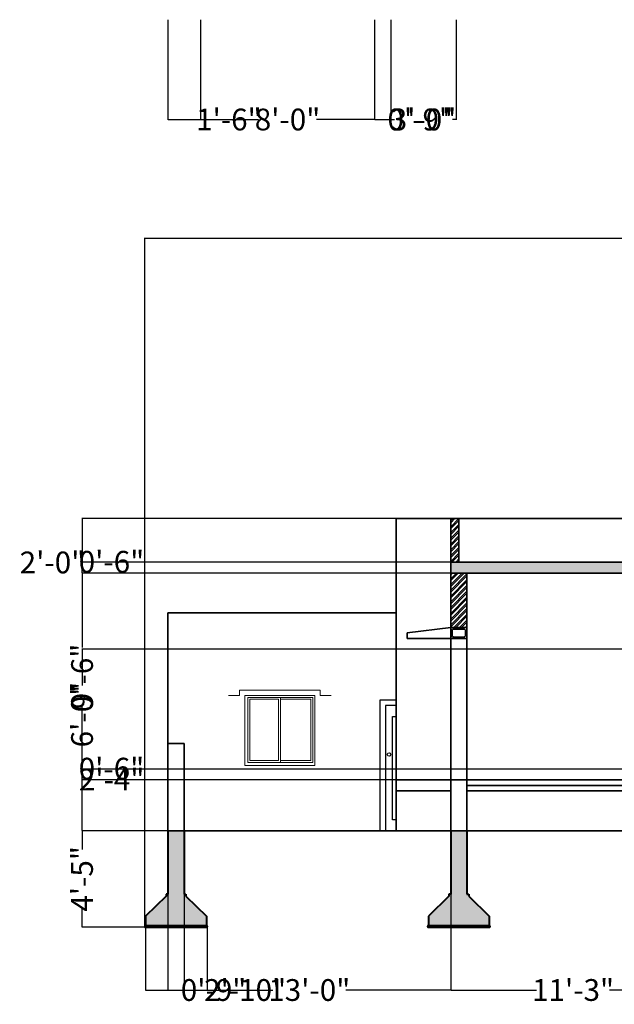
# Model space of a CAD drawing. Units: inches. Extents: x 1146 to 2917, y 889 to 2437.
# Tile 1 of 13: x 1223 to 1551, y 889 to 1432. Entities that reach past the tile are written whole.
import ezdxf

# ---------------------------------------------------------------- set-up
doc = ezdxf.new("R2010")
doc.units = ezdxf.units.IN
doc.header["$MEASUREMENT"] = 0
for name, color, linetype, lineweight in [('A-ANNO-DIMS', 2, 'Continuous', 18), ('A-SECT', 7, 'Continuous', 35), ('A-SECT-PATT', 8, 'Continuous', 13), ('door', 10, 'Continuous', 25), ('S-FNDN', 7, 'Continuous', 40), ('window', 5, 'Continuous', 18)]:
    doc.layers.add(name, color=color, linetype=linetype, lineweight=lineweight)
doc.styles.get("Standard").update_dxf_attribs({"font": 'arial.ttf'})
doc.dimstyles.get("Standard").update_dxf_attribs({"dimtxt": 12, "dimasz": 0.18, "dimexe": 0.18, "dimexo": 0.0625, "dimgap": 0.09, "dimtad": 0, "dimtoh": 1, "dimdec": 1, "dimzin": 0, "dimdsep": 46, "dimlunit": 4, "dimtxsty": 'Standard', "dimcen": 0.09, "dimadec": 0, "dimazin": 0, "dimtfac": 1, "dimtdec": 1, "dimtofl": 0, "dimtmove": 0, "dimatfit": 3, "dimfxl": 1, "dimtolj": 1, "dimtzin": 0, "dimarcsym": 0})
pattern_1 = [(50, (0, 0), (2.1517805, -0.1882564), [0.225, -2.475]), (355, (0, 0), (-0.416254, 2.2565764), [0.18, -1.98]), (100.45144, (0.1793, -0.0157), (1.7355265, 2.06832), [0.1912206, -2.1034263]), (46.1842, (0, 0.6), (3.201724, -0.496558), [0.3375, -3.7125]), (96.63564, (0.2668, 0.5586), (2.803986, 2.922356), [0.286831, -3.1551413]), (351.18416, (0, 0.6), (2.803986, 2.922356), [0.27, -2.97]), (21, (0.3, 0.45), (1.7907212, -1.2078567), [0.225, -2.475]), (326, (0.3, 0.45), (0.729946, 2.1754501), [0.18, -1.98]), (71.45144, (0.4492, 0.3493), (2.5206671, 0.9675935), [0.1912206, -2.1034263]), (37.5, (0, 0), (0.03647957, 0.99868156), [0, -1.956, 0, -2.01, 0, -1.9875]), (7.5, (0, 0), (0.7892086, 1.18323514), [0, -1.146, 0, -1.911, 0, -0.7575]), (327.5, (-0.669, 0), (1.6014673, -0.06766462), [0, -0.75, 0, -2.34, 0, -3.105]), (317.5, (-0.969, 0), (1.7495585, 0.30031495), [0, -0.975, 0, -1.554, 0, -2.205])]

# ---------------------------------------------------------------- blocks, each defined once
blk = doc.blocks.new('*D141')
at = {"layer": 'A-ANNO-DIMS', "color": 0, "lineweight": -2, "transparency": 16777216}
for p, q in [((1292.5, 931.94), (1292.5, 1311.7)), ((1292.68, 1311.52), (1597.13, 1311.52)), ((1970.95, 1311.52), (1666.5, 1311.52)), ((1971.13, 1277.03), (1971.13, 1311.7))]:
    blk.add_line(p, q, dxfattribs=at)
at = {"layer": 'A-ANNO-DIMS', "color": 0, "transparency": 16777216}
for points in [[(1292.68, 1311.55), (1292.68, 1311.49), (1292.5, 1311.52)], [(1970.95, 1311.55), (1970.95, 1311.49), (1971.13, 1311.52)]]:
    blk.add_solid(points, dxfattribs=at)
at = {"layer": 'Defpoints', "color": 0, "transparency": 16777216}
for p in [(1971.13, 1311.52), (1971.13, 1276.97), (1292.5, 931.87)]:
    blk.add_point(p, dxfattribs=at)
at = {"layer": 'A-ANNO-DIMS', "color": 0, "transparency": 16777216, "insert": (1631.82, 1311.52), "char_height": 12, "attachment_point": 5}
blk.add_mtext('\\A1;56\'-6 1/2"', dxfattribs=at)
blk = doc.blocks.new('*D143')
at = {"layer": 'A-ANNO-DIMS', "color": 0, "lineweight": -2, "transparency": 16777216}
for p, q in [((1431.07, 1012.97), (1257.62, 1012.97)), ((1257.8, 1012.97), (1257.8, 1013.15)), ((1257.8, 1013.15), (1257.98, 1013.15)), ((1257.8, 985.15), (1257.8, 1012.79)), ((1431.07, 984.97), (1257.62, 984.97))]:
    blk.add_line(p, q, dxfattribs=at)
at = {"layer": 'A-ANNO-DIMS', "color": 0, "transparency": 16777216}
for points in [[(1257.77, 1012.79), (1257.83, 1012.79), (1257.8, 1012.97)], [(1257.77, 985.15), (1257.83, 985.15), (1257.8, 984.97)]]:
    blk.add_solid(points, dxfattribs=at)
at = {"layer": 'Defpoints', "color": 0, "transparency": 16777216}
for p in [(1257.8, 1012.97), (1431.13, 1012.97), (1431.13, 984.97)]:
    blk.add_point(p, dxfattribs=at)
at = {"layer": 'A-ANNO-DIMS', "color": 0, "transparency": 16777216, "insert": (1274.12, 1013.15), "char_height": 12, "attachment_point": 5}
blk.add_mtext('\\A1;2\'-4"', dxfattribs=at)
blk = doc.blocks.new('*D144')
at = {"layer": 'A-ANNO-DIMS', "color": 0, "lineweight": -2, "transparency": 16777216}
for p, q in [((1470.07, 1126.97), (1257.62, 1126.97)), ((1257.8, 1126.79), (1257.8, 1086.01)), ((1257.8, 1013.15), (1257.8, 1053.93)), ((1470.07, 1012.97), (1257.62, 1012.97))]:
    blk.add_line(p, q, dxfattribs=at)
at = {"layer": 'A-ANNO-DIMS', "color": 0, "transparency": 16777216}
for points in [[(1257.77, 1126.79), (1257.83, 1126.79), (1257.8, 1126.97)], [(1257.77, 1013.15), (1257.83, 1013.15), (1257.8, 1012.97)]]:
    blk.add_solid(points, dxfattribs=at)
at = {"layer": 'Defpoints', "color": 0, "transparency": 16777216}
for p in [(1470.13, 1126.97), (1257.8, 1012.97), (1470.13, 1012.97)]:
    blk.add_point(p, dxfattribs=at)
at = {"layer": 'A-ANNO-DIMS', "color": 0, "transparency": 16777216, "insert": (1257.8, 1069.97), "char_height": 12, "attachment_point": 5, "rotation": 90}
blk.add_mtext('\\A1;9\'-6"', dxfattribs=at)
blk = doc.blocks.new('*D145')
at = {"layer": 'A-ANNO-DIMS', "color": 0, "lineweight": -2, "transparency": 16777216}
for p, q in [((1461.07, 1156.97), (1257.62, 1156.97)), ((1257.8, 1156.79), (1257.8, 1133.15)), ((1461.07, 1132.97), (1257.62, 1132.97)), ((1257.8, 1132.79), (1257.62, 1132.79)), ((1257.8, 1132.97), (1257.8, 1132.79))]:
    blk.add_line(p, q, dxfattribs=at)
at = {"layer": 'A-ANNO-DIMS', "color": 0, "transparency": 16777216}
for points in [[(1257.77, 1156.79), (1257.83, 1156.79), (1257.8, 1156.97)], [(1257.77, 1133.15), (1257.83, 1133.15), (1257.8, 1132.97)]]:
    blk.add_solid(points, dxfattribs=at)
at = {"layer": 'Defpoints', "color": 0, "transparency": 16777216}
for p in [(1461.13, 1156.97), (1257.8, 1132.97), (1461.13, 1132.97)]:
    blk.add_point(p, dxfattribs=at)
at = {"layer": 'A-ANNO-DIMS', "color": 0, "transparency": 16777216, "insert": (1241.48, 1132.79), "char_height": 12, "attachment_point": 5}
blk.add_mtext('\\A1;2\'-0"', dxfattribs=at)
blk = doc.blocks.new('*D146')
at = {"layer": 'A-ANNO-DIMS', "color": 0, "lineweight": -2, "transparency": 16777216}
for p, q in [((1305.13, 984.9), (1305.13, 897)), ((1461.13, 984.9), (1461.13, 897)), ((1305.31, 897.18), (1363, 897.18)), ((1460.95, 897.18), (1403.27, 897.18))]:
    blk.add_line(p, q, dxfattribs=at)
at = {"layer": 'A-ANNO-DIMS', "color": 0, "transparency": 16777216}
for points in [[(1305.31, 897.21), (1305.31, 897.15), (1305.13, 897.18)], [(1460.95, 897.21), (1460.95, 897.15), (1461.13, 897.18)]]:
    blk.add_solid(points, dxfattribs=at)
at = {"layer": 'Defpoints', "color": 0, "transparency": 16777216}
for p in [(1305.13, 984.97), (1461.13, 984.97), (1461.13, 897.18)]:
    blk.add_point(p, dxfattribs=at)
at = {"layer": 'A-ANNO-DIMS', "color": 0, "transparency": 16777216, "insert": (1383.13, 897.18), "char_height": 12, "attachment_point": 5}
blk.add_mtext('\\A1;13\'-0"', dxfattribs=at)
blk = doc.blocks.new('*D147')
at = {"layer": 'A-ANNO-DIMS', "color": 0, "lineweight": -2, "transparency": 16777216}
for p, q in [((1461.13, 984.9), (1461.13, 897)), ((1596.13, 984.9), (1596.13, 897)), ((1461.31, 897.18), (1508.5, 897.18)), ((1595.95, 897.18), (1548.77, 897.18))]:
    blk.add_line(p, q, dxfattribs=at)
at = {"layer": 'A-ANNO-DIMS', "color": 0, "transparency": 16777216}
for points in [[(1461.31, 897.21), (1461.31, 897.15), (1461.13, 897.18)], [(1595.95, 897.21), (1595.95, 897.15), (1596.13, 897.18)]]:
    blk.add_solid(points, dxfattribs=at)
at = {"layer": 'Defpoints', "color": 0, "transparency": 16777216}
for p in [(1461.13, 984.97), (1596.13, 984.97), (1596.13, 897.18)]:
    blk.add_point(p, dxfattribs=at)
at = {"layer": 'A-ANNO-DIMS', "color": 0, "transparency": 16777216, "insert": (1528.63, 897.18), "char_height": 12, "attachment_point": 5}
blk.add_mtext('\\A1;11\'-3"', dxfattribs=at)
blk = doc.blocks.new('*D150')
at = {"layer": 'A-ANNO-DIMS', "color": 0, "lineweight": -2, "transparency": 16777216}
for p, q in [((1305.07, 984.97), (1257.62, 984.97)), ((1257.8, 984.79), (1257.8, 974.7)), ((1257.8, 932.05), (1257.8, 942.14)), ((1292.44, 931.87), (1257.62, 931.87))]:
    blk.add_line(p, q, dxfattribs=at)
at = {"layer": 'A-ANNO-DIMS', "color": 0, "transparency": 16777216}
for points in [[(1257.77, 984.79), (1257.83, 984.79), (1257.8, 984.97)], [(1257.77, 932.05), (1257.83, 932.05), (1257.8, 931.87)]]:
    blk.add_solid(points, dxfattribs=at)
at = {"layer": 'Defpoints', "color": 0, "transparency": 16777216}
for p in [(1305.13, 984.97), (1257.8, 931.87), (1292.5, 931.87)]:
    blk.add_point(p, dxfattribs=at)
at = {"layer": 'A-ANNO-DIMS', "color": 0, "transparency": 16777216, "insert": (1257.8, 958.42), "char_height": 12, "attachment_point": 5, "rotation": 90}
blk.add_mtext('\\A1;4\'-5"', dxfattribs=at)
blk = doc.blocks.new('*D154')
at = {"layer": 'A-ANNO-DIMS', "color": 0, "lineweight": -2, "transparency": 16777216}
for p, q in [((1830.07, 1018.97), (1257.62, 1018.97)), ((1257.8, 1018.97), (1257.8, 1019.15)), ((1257.8, 1019.15), (1257.98, 1019.15)), ((1257.8, 1013.15), (1257.8, 1018.79)), ((1830.07, 1012.97), (1257.62, 1012.97))]:
    blk.add_line(p, q, dxfattribs=at)
at = {"layer": 'A-ANNO-DIMS', "color": 0, "transparency": 16777216}
for points in [[(1257.77, 1018.79), (1257.83, 1018.79), (1257.8, 1018.97)], [(1257.77, 1013.15), (1257.83, 1013.15), (1257.8, 1012.97)]]:
    blk.add_solid(points, dxfattribs=at)
at = {"layer": 'Defpoints', "color": 0, "transparency": 16777216}
for p in [(1257.8, 1018.97), (1830.13, 1018.97), (1830.13, 1012.97)]:
    blk.add_point(p, dxfattribs=at)
at = {"layer": 'A-ANNO-DIMS', "color": 0, "transparency": 16777216, "insert": (1274.02, 1019.15), "char_height": 12, "attachment_point": 5}
blk.add_mtext('\\A1;0\'-6"', dxfattribs=at)
blk = doc.blocks.new('*D157')
at = {"layer": 'A-ANNO-DIMS', "color": 0, "lineweight": -2, "transparency": 16777216}
for p, q in [((1830.07, 1084.97), (1257.62, 1084.97)), ((1257.8, 1084.79), (1257.8, 1065.04)), ((1257.8, 1013.15), (1257.8, 1032.89)), ((1830.07, 1012.97), (1257.62, 1012.97))]:
    blk.add_line(p, q, dxfattribs=at)
at = {"layer": 'A-ANNO-DIMS', "color": 0, "transparency": 16777216}
for points in [[(1257.77, 1084.79), (1257.83, 1084.79), (1257.8, 1084.97)], [(1257.77, 1013.15), (1257.83, 1013.15), (1257.8, 1012.97)]]:
    blk.add_solid(points, dxfattribs=at)
at = {"layer": 'Defpoints', "color": 0, "transparency": 16777216}
for p in [(1257.8, 1084.97), (1830.13, 1084.97), (1830.13, 1012.97)]:
    blk.add_point(p, dxfattribs=at)
at = {"layer": 'A-ANNO-DIMS', "color": 0, "transparency": 16777216, "insert": (1257.8, 1048.97), "char_height": 12, "attachment_point": 5, "rotation": 90}
blk.add_mtext('\\A1;6\'-0"', dxfattribs=at)
blk = doc.blocks.new('*D158')
at = {"layer": 'A-ANNO-DIMS', "color": 0, "lineweight": -2, "transparency": 16777216}
for p, q in [((1461.07, 1132.97), (1257.62, 1132.97)), ((1257.8, 1132.97), (1257.8, 1133.15)), ((1257.8, 1133.15), (1257.98, 1133.15)), ((1257.8, 1127.15), (1257.8, 1132.79)), ((1461.07, 1126.97), (1257.62, 1126.97))]:
    blk.add_line(p, q, dxfattribs=at)
at = {"layer": 'A-ANNO-DIMS', "color": 0, "transparency": 16777216}
for points in [[(1257.77, 1132.79), (1257.83, 1132.79), (1257.8, 1132.97)], [(1257.77, 1127.15), (1257.83, 1127.15), (1257.8, 1126.97)]]:
    blk.add_solid(points, dxfattribs=at)
at = {"layer": 'Defpoints', "color": 0, "transparency": 16777216}
for p in [(1257.8, 1132.97), (1461.13, 1132.97), (1461.13, 1126.97)]:
    blk.add_point(p, dxfattribs=at)
at = {"layer": 'A-ANNO-DIMS', "color": 0, "transparency": 16777216, "insert": (1274.02, 1133.15), "char_height": 12, "attachment_point": 5}
blk.add_mtext('\\A1;0\'-6"', dxfattribs=at)
blk = doc.blocks.new('*D159')
at = {"layer": 'A-ANNO-DIMS', "color": 0, "lineweight": -2, "transparency": 16777216}
for p, q in [((1292.85, 932.16), (1292.85, 897)), ((1326.77, 931.81), (1326.77, 897)), ((1293.03, 897.18), (1326.59, 897.18)), ((1326.77, 897.18), (1326.95, 897.18))]:
    blk.add_line(p, q, dxfattribs=at)
at = {"layer": 'A-ANNO-DIMS', "color": 0, "transparency": 16777216}
for points in [[(1293.03, 897.21), (1293.03, 897.15), (1292.85, 897.18)], [(1326.59, 897.21), (1326.59, 897.15), (1326.77, 897.18)]]:
    blk.add_solid(points, dxfattribs=at)
at = {"layer": 'Defpoints', "color": 0, "transparency": 16777216}
for p in [(1292.85, 932.23), (1326.77, 931.87), (1326.77, 897.18)]:
    blk.add_point(p, dxfattribs=at)
at = {"layer": 'A-ANNO-DIMS', "color": 0, "transparency": 16777216, "insert": (1347.75, 897.18), "char_height": 12, "attachment_point": 5}
blk.add_mtext('\\A1;2\'-10"', dxfattribs=at)
blk = doc.blocks.new('*D160')
at = {"layer": 'A-ANNO-DIMS', "color": 0, "lineweight": -2, "transparency": 16777216}
for p, q in [((1305.13, 984.9), (1305.13, 897)), ((1314.13, 984.9), (1314.13, 897)), ((1305.31, 897.18), (1313.95, 897.18)), ((1314.13, 897.18), (1314.31, 897.18))]:
    blk.add_line(p, q, dxfattribs=at)
at = {"layer": 'A-ANNO-DIMS', "color": 0, "transparency": 16777216}
for points in [[(1305.31, 897.21), (1305.31, 897.15), (1305.13, 897.18)], [(1313.95, 897.21), (1313.95, 897.15), (1314.13, 897.18)]]:
    blk.add_solid(points, dxfattribs=at)
at = {"layer": 'Defpoints', "color": 0, "transparency": 16777216}
for p in [(1305.13, 984.97), (1314.13, 984.97), (1314.13, 897.18)]:
    blk.add_point(p, dxfattribs=at)
at = {"layer": 'A-ANNO-DIMS', "color": 0, "transparency": 16777216, "insert": (1330.35, 897.18), "char_height": 12, "attachment_point": 5}
blk.add_mtext('\\A1;0\'-9"', dxfattribs=at)
blk = doc.blocks.new('*D162')
at = {"layer": 'A-ANNO-DIMS', "color": 0, "lineweight": -2, "transparency": 16777216}
for p, q in [((1305.13, 1431.83), (1305.13, 1376.71)), ((1323.13, 1431.83), (1323.13, 1376.71)), ((1305.31, 1376.89), (1322.95, 1376.89)), ((1323.13, 1376.89), (1323.31, 1376.89))]:
    blk.add_line(p, q, dxfattribs=at)
at = {"layer": 'A-ANNO-DIMS', "color": 0, "transparency": 16777216}
for points in [[(1305.31, 1376.92), (1305.31, 1376.86), (1305.13, 1376.89)], [(1322.95, 1376.92), (1322.95, 1376.86), (1323.13, 1376.89)]]:
    blk.add_solid(points, dxfattribs=at)
at = {"layer": 'Defpoints', "color": 0, "transparency": 16777216}
for p in [(1305.13, 1431.89), (1323.13, 1431.89), (1323.13, 1376.89)]:
    blk.add_point(p, dxfattribs=at)
at = {"layer": 'A-ANNO-DIMS', "color": 0, "transparency": 16777216, "insert": (1338.79, 1376.89), "char_height": 12, "attachment_point": 5}
blk.add_mtext('\\A1;1\'-6"', dxfattribs=at)
blk = doc.blocks.new('*D163')
at = {"layer": 'A-ANNO-DIMS', "color": 0, "lineweight": -2, "transparency": 16777216}
for p, q in [((1323.13, 1431.83), (1323.13, 1376.71)), ((1419.13, 1431.83), (1419.13, 1376.71)), ((1323.31, 1376.89), (1355.09, 1376.89)), ((1418.95, 1376.89), (1387.18, 1376.89))]:
    blk.add_line(p, q, dxfattribs=at)
at = {"layer": 'A-ANNO-DIMS', "color": 0, "transparency": 16777216}
for points in [[(1323.31, 1376.92), (1323.31, 1376.86), (1323.13, 1376.89)], [(1418.95, 1376.92), (1418.95, 1376.86), (1419.13, 1376.89)]]:
    blk.add_solid(points, dxfattribs=at)
at = {"layer": 'Defpoints', "color": 0, "transparency": 16777216}
for p in [(1323.13, 1431.89), (1419.13, 1431.89), (1419.13, 1376.89)]:
    blk.add_point(p, dxfattribs=at)
at = {"layer": 'A-ANNO-DIMS', "color": 0, "transparency": 16777216, "insert": (1371.13, 1376.89), "char_height": 12, "attachment_point": 5}
blk.add_mtext('\\A1;8\'-0"', dxfattribs=at)
blk = doc.blocks.new('*D164')
at = {"layer": 'A-ANNO-DIMS', "color": 0, "lineweight": -2, "transparency": 16777216}
for p, q in [((1419.13, 1431.83), (1419.13, 1376.71)), ((1428.13, 1431.83), (1428.13, 1376.71)), ((1419.31, 1376.89), (1427.95, 1376.89)), ((1428.13, 1376.89), (1428.31, 1376.89))]:
    blk.add_line(p, q, dxfattribs=at)
at = {"layer": 'A-ANNO-DIMS', "color": 0, "transparency": 16777216}
for points in [[(1419.31, 1376.92), (1419.31, 1376.86), (1419.13, 1376.89)], [(1427.95, 1376.92), (1427.95, 1376.86), (1428.13, 1376.89)]]:
    blk.add_solid(points, dxfattribs=at)
at = {"layer": 'Defpoints', "color": 0, "transparency": 16777216}
for p in [(1419.13, 1431.89), (1428.13, 1431.89), (1428.13, 1376.89)]:
    blk.add_point(p, dxfattribs=at)
at = {"layer": 'A-ANNO-DIMS', "color": 0, "transparency": 16777216, "insert": (1444.35, 1376.89), "char_height": 12, "attachment_point": 5}
blk.add_mtext('\\A1;0\'-9"', dxfattribs=at)
blk = doc.blocks.new('*D165')
at = {"layer": 'A-ANNO-DIMS', "color": 0, "lineweight": -2, "transparency": 16777216}
for p, q in [((1428.13, 1431.83), (1428.13, 1376.71)), ((1464.13, 1431.83), (1464.13, 1376.71)), ((1428.31, 1376.89), (1430.1, 1376.89)), ((1463.95, 1376.89), (1462.17, 1376.89))]:
    blk.add_line(p, q, dxfattribs=at)
at = {"layer": 'A-ANNO-DIMS', "color": 0, "transparency": 16777216}
for points in [[(1428.31, 1376.92), (1428.31, 1376.86), (1428.13, 1376.89)], [(1463.95, 1376.92), (1463.95, 1376.86), (1464.13, 1376.89)]]:
    blk.add_solid(points, dxfattribs=at)
at = {"layer": 'Defpoints', "color": 0, "transparency": 16777216}
for p in [(1428.13, 1431.89), (1464.13, 1431.89), (1464.13, 1376.89)]:
    blk.add_point(p, dxfattribs=at)
at = {"layer": 'A-ANNO-DIMS', "color": 0, "transparency": 16777216, "insert": (1446.13, 1376.89), "char_height": 12, "attachment_point": 5}
blk.add_mtext('\\A1;3\'-0"', dxfattribs=at)

msp = doc.modelspace()

# ---------------------------------------------------------------- hatches: boundary and pattern name
at = {"layer": 'A-SECT-PATT'}
h = msp.add_hatch(dxfattribs=at)
h.set_pattern_fill('ANSI32', color=256, scale=6)
h.paths.add_polyline_path([(1605.13, 1126.97), (1596.13, 1126.97), (1596.13, 1102.97), (1605.13, 1102.97)])
h.paths.add_polyline_path([(1794.13, 1126.97), (1785.13, 1126.97), (1785.13, 1102.97), (1794.13, 1102.97)])
h.paths.add_polyline_path([(1470.13, 1126.97), (1461.13, 1126.97), (1461.13, 1096.97), (1470.13, 1096.97)])
h.paths.add_polyline_path([(1461.13, 1132.97), (1465.63, 1132.97), (1465.63, 1156.97), (1461.13, 1156.97)])
h = msp.add_hatch(dxfattribs=at)
h.set_pattern_fill('AR-CONC', color=256, scale=0.3)
h.set_pattern_definition(pattern_1)
h.paths.add_polyline_path([(1856.99, 1126.97), (1856.99, 1132.97), (1461.13, 1132.97), (1461.13, 1126.97)])
h = msp.add_hatch(dxfattribs=at)
h.set_pattern_fill('AR-CONC', color=256, scale=0.3)
h.set_pattern_definition(pattern_1)
h.paths.add_polyline_path([(1315.13, 948.97), (1315.13, 949.97), (1314.13, 949.97), (1314.13, 984.97), (1305.13, 984.97), (1305.13, 949.97), (1304.13, 949.97), (1304.13, 948.97), (1292.85, 937.8), (1292.85, 932.73), (1326.42, 932.73), (1326.42, 937.8)])
h = msp.add_hatch(dxfattribs=at)
h.set_pattern_fill('AR-CONC', color=256, scale=0.3)
h.set_pattern_definition([(50, (156, 0), (2.1517805, -0.1882564), [0.225, -2.475]), (355, (156, 0), (-0.416254, 2.2565764), [0.18, -1.98]), (100.45144, (156.1793, -0.0157), (1.7355265, 2.06832), [0.1912206, -2.1034263]), (46.1842, (156, 0.6), (3.201724, -0.496558), [0.3375, -3.7125]), (96.63564, (156.2668, 0.5586), (2.803986, 2.922356), [0.286831, -3.155141]), (351.18416, (156, 0.6), (2.803986, 2.922356), [0.27, -2.97]), (21, (156.3, 0.45), (1.7907212, -1.2078567), [0.225, -2.475]), (326, (156.3, 0.45), (0.729946, 2.17545), [0.18, -1.98]), (71.45144, (156.4492, 0.3493), (2.520667, 0.9675935), [0.1912206, -2.1034263]), (37.5, (156, 0), (0.03647957, 0.99868156), [0, -1.956, 0, -2.01, 0, -1.9875]), (7.5, (156, 0), (0.7892086, 1.18323514), [0, -1.146, 0, -1.911, 0, -0.7575]), (327.5, (155.331, 0), (1.6014673, -0.0676646), [0, -0.75, 0, -2.34, 0, -3.105]), (317.5, (155.031, 0), (1.7495585, 0.300315), [0, -0.975, 0, -1.554, 0, -2.205])])
h.paths.add_polyline_path([(1471.13, 948.97), (1471.13, 949.97), (1470.13, 949.97), (1470.13, 984.97), (1461.13, 984.97), (1461.13, 949.97), (1460.13, 949.97), (1460.13, 948.97), (1448.85, 937.8), (1448.85, 932.73), (1482.42, 932.73), (1482.42, 937.8)])

# ---------------------------------------------------------------- linework, layer by layer
at = {"layer": 'A-SECT'}
for p, q in [((1461.13, 1156.97), (1431.13, 1156.97)), ((1431.13, 1132.97), (1431.13, 1156.97)), ((1461.13, 1156.97), (1785.13, 1156.97)), ((1461.13, 1126.97), (1461.13, 1156.97)), ((1465.63, 1132.97), (1465.63, 1156.97)), ((1431.13, 1132.97), (1431.13, 984.97)), ((1461.13, 1132.97), (1856.99, 1132.97)), ((1461.13, 984.97), (1461.13, 1126.97)), ((1461.13, 1126.97), (1856.99, 1126.97)), ((1470.13, 984.97), (1470.13, 1126.97)), ((1305.13, 984.97), (1305.13, 1104.97)), ((1305.13, 1104.97), (1431.13, 1104.97)), ((1437.13, 1093.97), (1461.13, 1096.97)), ((1470.13, 1096.97), (1461.13, 1096.97)), ((1437.13, 1090.97), (1437.13, 1093.97)), ((1461.13, 1090.97), (1437.13, 1090.97)), ((1470.13, 1090.97), (1461.13, 1090.97)), ((1305.13, 1032.97), (1314.13, 1032.97)), ((1314.13, 984.97), (1314.13, 1032.97)), ((1638.13, 1012.97), (1431.13, 1012.97)), ((1470.13, 1012.97), (1971.13, 1012.97)), ((1470.13, 1009.97), (1596.13, 1009.97)), ((1431.13, 1006.97), (1461.13, 1006.97)), ((1470.13, 1006.97), (1596.13, 1006.97)), ((1305.13, 984.97), (1314.13, 984.97)), ((1314.13, 984.97), (1461.13, 984.97)), ((1461.13, 984.97), (1971.13, 984.97))]:
    msp.add_line(p, q, dxfattribs=at)
msp.add_lwpolyline([(1462.92, 1096.05), (1468.31, 1096.05, -0.414214), (1469.31, 1095.05), (1469.31, 1092.71, -0.414214), (1468.31, 1091.71), (1462.92, 1091.71, -0.414214), (1461.92, 1092.71), (1461.92, 1095.05, -0.414214)], format="xyb", close=True, dxfattribs=at)
at = {"layer": 'door'}
for points in [[(1431.13, 1056.97), (1422.13, 1056.97), (1422.13, 984.97), (1425.13, 984.97)], [(1431.13, 1053.94), (1425.13, 1053.94), (1425.13, 984.97), (1455.13, 984.97)], [(1431.13, 990.97), (1429.13, 990.97), (1429.13, 1047.94), (1431.13, 1047.94)], [(1455.13, 984.97), (1458.13, 984.97)]]:
    msp.add_lwpolyline(points, dxfattribs=at)
msp.add_circle((1427.13, 1026.97), 1, dxfattribs=at)
at = {"layer": 'S-FNDN'}
for p, q in [((1305.13, 984.97), (1305.13, 949.97)), ((1314.13, 984.97), (1314.13, 949.97)), ((1461.13, 984.97), (1461.13, 949.97)), ((1470.13, 984.97), (1470.13, 949.97)), ((1305.13, 949.97), (1304.13, 949.97)), ((1304.13, 949.97), (1304.13, 948.97)), ((1314.13, 949.97), (1315.13, 949.97)), ((1315.13, 949.97), (1315.13, 948.97)), ((1461.13, 949.97), (1460.13, 949.97)), ((1460.13, 949.97), (1460.13, 948.97)), ((1470.13, 949.97), (1471.13, 949.97)), ((1471.13, 949.97), (1471.13, 948.97)), ((1304.13, 948.97), (1292.85, 937.8)), ((1315.13, 948.97), (1326.42, 937.8)), ((1460.13, 948.97), (1448.85, 937.8)), ((1471.13, 948.97), (1482.42, 937.8)), ((1292.85, 937.8), (1292.85, 932.73)), ((1326.42, 937.8), (1326.42, 932.73)), ((1448.85, 937.8), (1448.85, 932.73)), ((1482.42, 937.8), (1482.42, 932.73)), ((1292.85, 932.73), (1326.42, 932.73)), ((1292.85, 931.73), (1326.42, 931.73)), ((1448.85, 932.73), (1482.42, 932.73)), ((1448.85, 931.73), (1482.42, 931.73))]:
    msp.add_line(p, q, dxfattribs=at)
for centre, start, end in [((1292.85, 932.23), 90, 270), ((1326.42, 932.23), 270, 90), ((1448.85, 932.23), 90, 270), ((1482.42, 932.23), 270, 90)]:
    msp.add_arc(centre, 0.5, start, end, dxfattribs=at)
at = {"layer": 'window'}
for p, q in [((1344.63, 1059.47), (1338.63, 1059.47)), ((1349.26, 1022.6), (1349.26, 1058.45)), ((1349.26, 1058.45), (1367.19, 1058.45)), ((1367.19, 1022.6), (1367.19, 1058.45)), ((1367.19, 1058.45), (1385.12, 1058.45)), ((1385.12, 1058.45), (1385.12, 1022.6)), ((1389.13, 1059.47), (1395.13, 1059.47)), ((1367.19, 1022.6), (1349.26, 1022.6)), ((1385.12, 1022.6), (1367.19, 1022.6))]:
    msp.add_line(p, q, dxfattribs=at)
for points in [[(1389.13, 1059.47), (1389.13, 1062.47), (1344.63, 1062.47), (1344.63, 1059.47)], [(1366.11, 1057.37), (1366.11, 1023.68), (1350.35, 1023.68), (1350.35, 1057.37), (1366.11, 1057.37)], [(1367.19, 1057.37), (1384.03, 1057.37), (1384.03, 1023.68), (1367.19, 1023.68)]]:
    msp.add_lwpolyline(points, dxfattribs=at)
msp.add_lwpolyline([(1347.63, 1020.97), (1386.13, 1020.97), (1386.13, 1059.47), (1347.63, 1059.47)], close=True, dxfattribs=at)

# ---------------------------------------------------------------- dimensions: what is measured, and where the dimension line sits
at = {"layer": 'A-ANNO-DIMS'}
for base, p1, p2, picture, middle in [((1323.13, 1376.89), (1305.13, 1431.89), (1323.13, 1431.89), '*D162', (1338.79, 1376.89)), ((1419.13, 1376.89), (1323.13, 1431.89), (1419.13, 1431.89), '*D163', (1371.13, 1376.89)), ((1428.13, 1376.89), (1419.13, 1431.89), (1428.13, 1431.89), '*D164', (1444.35, 1376.89)), ((1464.13, 1376.89), (1428.13, 1431.89), (1464.13, 1431.89), '*D165', (1446.13, 1376.89)), ((1971.13, 1311.52), (1292.5, 931.87), (1971.13, 1276.97), '*D141', (1631.82, 1311.52)), ((1461.13, 897.18), (1305.13, 984.97), (1461.13, 984.97), '*D146', (1383.13, 897.18)), ((1314.13, 897.18), (1305.13, 984.97), (1314.13, 984.97), '*D160', (1330.35, 897.18)), ((1596.13, 897.18), (1461.13, 984.97), (1596.13, 984.97), '*D147', (1528.63, 897.18)), ((1326.77, 897.18), (1292.85, 932.23), (1326.77, 931.87), '*D159', (1347.75, 897.18))]:
    dim = msp.add_linear_dim(base=base, p1=p1, p2=p2, dimstyle='Standard', override={"dimdec": 1, "dimlfac": 1, "dimrnd": 0, "dimzin": 1, "dimdsep": 46, "dimlunit": 4, "dimfrac": 2}, dxfattribs=at)
    dim.commit()
    dim.dimension.update_dxf_attribs({"geometry": picture, "text_midpoint": middle})
for base, p1, p2, picture, middle in [((1257.8, 1132.97), (1461.13, 1156.97), (1461.13, 1132.97), '*D145', (1241.48, 1132.79)), ((1257.8, 1132.97), (1461.13, 1126.97), (1461.13, 1132.97), '*D158', (1274.02, 1133.15)), ((1257.8, 1012.97), (1470.13, 1126.97), (1470.13, 1012.97), '*D144', (1257.8, 1069.97)), ((1257.8, 1084.97), (1830.13, 1012.97), (1830.13, 1084.97), '*D157', (1257.8, 1048.97)), ((1257.8, 1018.97), (1830.13, 1012.97), (1830.13, 1018.97), '*D154', (1274.02, 1019.15)), ((1257.8, 1012.97), (1431.13, 984.97), (1431.13, 1012.97), '*D143', (1274.12, 1013.15)), ((1257.8, 931.87), (1305.13, 984.97), (1292.5, 931.87), '*D150', (1257.8, 958.42))]:
    dim = msp.add_linear_dim(base=base, p1=p1, p2=p2, angle=90, dimstyle='Standard', override={"dimdec": 1, "dimlfac": 1, "dimrnd": 0, "dimzin": 1, "dimdsep": 46, "dimlunit": 4, "dimfrac": 2}, dxfattribs=at)
    dim.commit()
    dim.dimension.update_dxf_attribs({"geometry": picture, "text_midpoint": middle})

doc.saveas('drawing.dxf')
